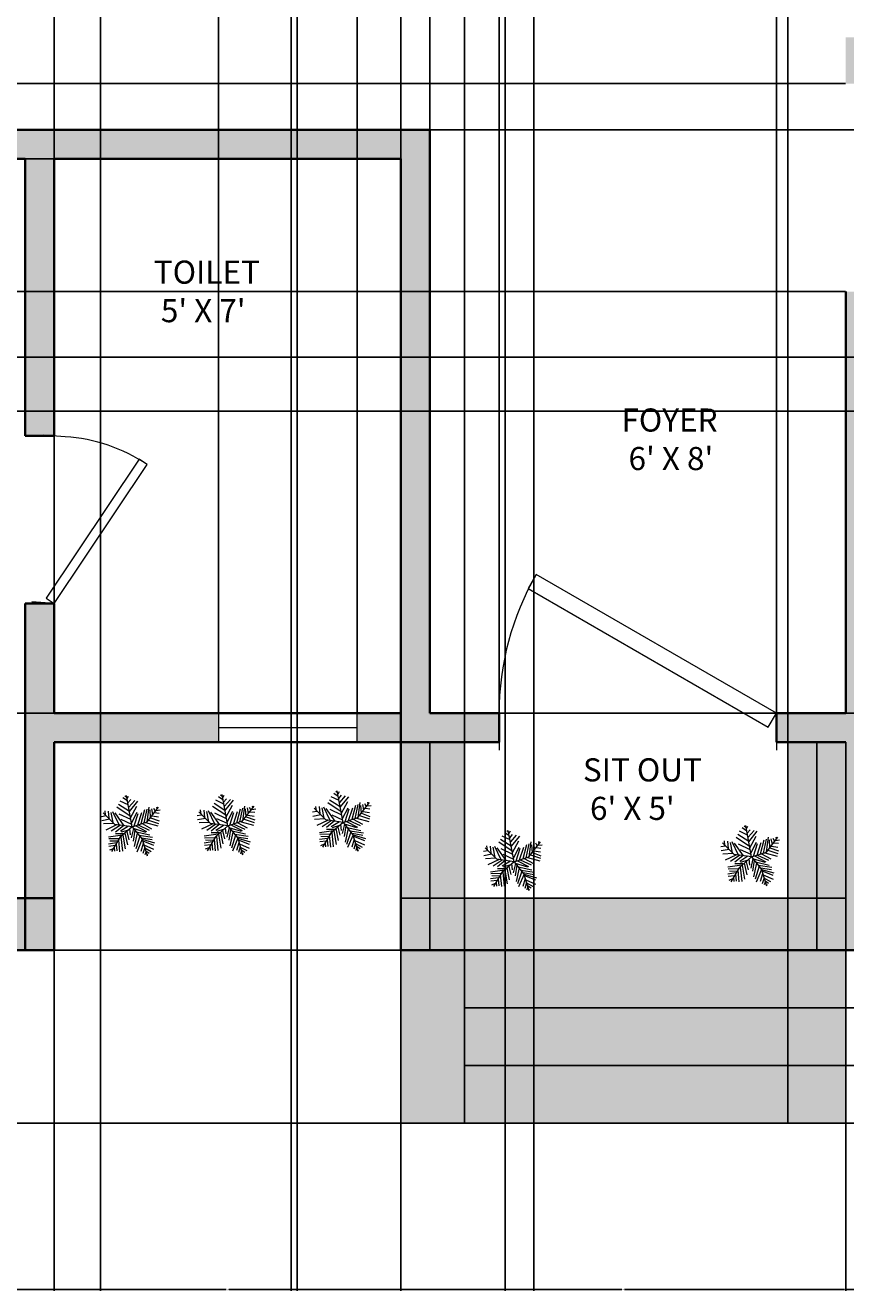
# Model space of a CAD drawing. Units: inches. Extents: x -28 to 649, y -11 to 509.
# Tile 2 of 7: x 204 to 346, y -11 to 208. Entities that reach past the tile are written whole.
import ezdxf

# ---------------------------------------------------------------- set-up
doc = ezdxf.new("R2010")
doc.units = ezdxf.units.IN
doc.header["$MEASUREMENT"] = 0
for name, color, linetype, lineweight in [('A-ANNO-DIMS', 2, 'Continuous', 18), ('A-AREA-IDEN', 18, 'Continuous', 18), ('A-FLOR-CURB-PATT', 31, 'Continuous', 13), ('A-FLOR-STRS', 7, 'Continuous', 25), ('A-FLOR-STRS-PATT', 254, 'Continuous', 13), ('A-WALL', 7, 'Continuous', 35), ('A-WALL-PATT', 251, 'Continuous', 13), ('doors', 40, 'Continuous', 20), ('L-PLNT', 90, 'Continuous', 13), ('window', 30, 'Continuous', 18)]:
    doc.layers.add(name, color=color, linetype=linetype, lineweight=lineweight)
doc.styles.get("Standard").update_dxf_attribs({"font": 'arial.ttf'})
doc.dimstyles.get("Standard").update_dxf_attribs({"dimtxt": 0.18, "dimasz": 0.18, "dimexe": 0.18, "dimexo": 0.0625, "dimgap": 0.09, "dimtad": 0, "dimtih": 1, "dimtoh": 1, "dimdec": 4, "dimzin": 0, "dimdsep": 46, "dimtxsty": 'Standard', "dimcen": 0.09, "dimadec": 0, "dimazin": 0, "dimtfac": 1, "dimtdec": 4, "dimtofl": 0, "dimtmove": 0, "dimatfit": 3, "dimfxl": 1, "dimtolj": 1, "dimtzin": 0, "dimarcsym": 0})

# ---------------------------------------------------------------- blocks, each defined once
blk = doc.blocks.new('*U10')
for p, q in [((0, 0), (0, 100)), ((750, 0), (750, 100))]:
    blk.add_line(p, q)
blk.add_lwpolyline([(0, 0), (649.5, -375), (671.4, -337.1), (21.9, 37.9)], close=True)
blk.add_arc((0, 0), 750, 330, 0)
blk = doc.blocks.new('*U2')
for p, q in [((-185.1152, 1008.5578), (-553.1612, 1185.4942)), ((-221.9198, 1197.3052), (-433.5526, 1338.8594)), ((-258.7244, 1362.456), (-332.3336, 1421.4348)), ((0, 0), (-266.7, 1447.8)), ((-231.1146, 1315.2628), (-166.7002, 1421.4348)), ((-194.31, 1102.9442), (-65.4812, 1256.284)), ((-148.3106, 914.1968), (118.5418, 1220.9018)), ((-129.8956, 701.8528), (265.7602, 1185.4942)), ((-800.1, 114.3), (-1333.5, 647.7)), ((-1234.059, 536.7274), (-1252.4486, 737.2604)), ((-1105.2302, 725.4494), (-1077.6458, 395.1732)), ((-976.4268, 666.4706), (-884.4026, 194.6402)), ((-902.8176, 713.6638), (-617.5756, 100.2538)), ((-369.1382, 53.086), (-783.1836, 642.874)), ((-93.091, 489.5342), (-700.3796, 902.3858)), ((-129.8956, 713.6638), (-626.7704, 1032.1544)), ((-617.5756, 607.4918), (-74.7014, 347.98)), ((-74.7014, 418.7444), (219.7608, 961.39)), ((-28.6766, 171.0436), (228.9556, 678.2816)), ((100.1268, 41.275), (284.1498, 619.2774)), ((256.5654, 88.4682), (449.7832, 666.4706)), ((412.9786, 147.447), (587.8068, 796.2392)), ((560.197, 182.8292), (698.2206, 819.8358)), ((685.8, 228.6), (1219.2, 914.4)), ((689.0258, 230.0224), (790.2448, 914.1968)), ((808.6344, 784.4282), (827.0494, 418.7444)), ((891.4384, 831.6214), (946.658, 572.1096)), ((983.4626, 867.0036), (1066.2666, 725.4494)), ((1029.462, 654.685), (1241.0948, 631.0884)), ((1112.2914, 760.8316), (1296.3144, 784.4282)), ((1121.4862, 925.9824), (1149.0706, 831.6214)), ((-1206.4492, 501.3198), (-1418.082, 465.9376)), ((-1031.621, 347.98), (-1399.667, 277.1902)), ((-847.598, 159.2326), (-1326.0578, 135.636)), ((-718.7946, 88.4682), (-1215.644, -147.447)), ((-543.9664, 76.6572), (-967.2066, -206.4512)), ((0, 0), (-800.1, 114.3)), ((-405.9428, 53.086), (-764.794, -241.8334)), ((0, 0), (-571.5, -495.3)), ((-166.7002, 29.4894), (-543.9664, -206.4512)), ((-525.5514, 347.98), (-28.6766, 123.8504)), ((0, 0), (685.8, 228.6)), ((0, 0), (457.2, -571.5)), ((164.5412, 41.275), (661.416, -218.2368)), ((284.1498, 88.4682), (781.0246, -147.447)), ((458.978, 147.447), (891.4384, -88.4682)), ((615.4166, 194.6402), (1185.8752, 41.275)), ((753.4148, 312.5978), (1222.6798, 159.2326)), ((845.439, 418.7444), (1241.0948, 277.1902)), ((919.0482, 501.3198), (1222.6798, 454.152)), ((-442.7474, -383.3876), (-1086.8406, -477.7486)), ((-617.5756, -548.5384), (-1077.6458, -560.324)), ((-571.5, -495.3), (-952.5, -1143)), ((-387.5278, -324.4088), (-764.794, -324.4088)), ((-525.5514, -465.963), (-451.9422, -1126.5408)), ((-166.7002, -147.447), (-507.1618, -253.619)), ((-433.5526, -383.3876), (-323.1134, -1020.3688)), ((-341.5284, -289.0012), (-221.9198, -831.6214)), ((-240.3094, -218.2368), (-157.5054, -595.7062)), ((-120.7008, -88.4682), (-93.091, -371.5766)), ((63.3222, -76.6826), (-37.8714, -513.1308)), ((44.9326, -64.897), (615.4166, -241.8334)), ((127.7366, -159.258), (54.1274, -654.685)), ((228.9556, -289.0012), (90.932, -914.1968)), ((357.759, -430.5554), (164.5412, -1020.3688)), ((192.151, -230.0224), (817.8292, -371.5766)), ((458.978, -572.1096), (210.5406, -1161.923)), ((311.7596, -383.3876), (937.4378, -477.7486)), ((412.9786, -501.3452), (919.0482, -583.9206)), ((457.2, -571.5), (685.8, -1333.5)), ((468.1982, -572.1096), (1029.462, -737.2604)), ((-718.7946, -737.2604), (-1086.8406, -796.2392)), ((-783.1836, -867.029), (-1077.6458, -902.4112)), ((-875.2078, -1008.5832), (-1040.8412, -1079.3476)), ((-681.9646, -666.496), (-1022.4262, -654.685)), ((-829.2084, -937.7934), (-810.7934, -1126.5408)), ((-737.1842, -784.4536), (-709.5744, -1114.7298)), ((-635.9652, -607.5172), (-580.771, -1150.1374)), ((514.1976, -772.6426), (403.7838, -1138.3264)), ((486.5878, -642.8994), (983.4626, -843.4324)), ((578.612, -961.39), (495.7826, -1232.7128)), ((541.8074, -831.6214), (992.6574, -1032.1544)), ((578.612, -973.1756), (873.0488, -1138.3264)), ((624.6114, -1161.923), (587.8068, -1291.6916)), ((624.6114, -1102.9442), (781.0246, -1209.1162)), ((679.8056, -1268.095), (716.6102, -1291.6916))]:
    blk.add_line(p, q)
blk = doc.blocks.new('*D31')
at = {"layer": 'A-ANNO-DIMS', "color": 0, "lineweight": -2, "transparency": 16777216}
for p, q in [((603.51, 479.94), (632.43, 479.94)), ((632.25, 479.76), (632.25, 249.12)), ((632.25, 18.12), (632.25, 248.76)), ((346.51, 17.94), (632.43, 17.94))]:
    blk.add_line(p, q, dxfattribs=at)
at = {"layer": 'A-ANNO-DIMS', "color": 0, "transparency": 16777216}
for points in [[(632.22, 479.76), (632.28, 479.76), (632.25, 479.94)], [(632.22, 18.12), (632.28, 18.12), (632.25, 17.94)]]:
    blk.add_solid(points, dxfattribs=at)
at = {"layer": 'Defpoints', "color": 0, "transparency": 16777216}
for p in [(603.45, 479.94), (632.25, 479.94), (346.45, 17.94)]:
    blk.add_point(p, dxfattribs=at)
at = {"layer": 'A-ANNO-DIMS', "color": 0, "transparency": 16777216, "insert": (632.25, 248.94), "char_height": 0.18, "attachment_point": 5}
blk.add_mtext('\\A1;462', dxfattribs=at)
blk = doc.blocks.new('*D32')
at = {"layer": 'A-ANNO-DIMS', "color": 0, "lineweight": -2, "transparency": 16777216}
for p, q in [((269.39, 47.94), (-1.53, 47.94)), ((-1.35, 47.76), (-1.35, 33.12)), ((-1.35, 18.12), (-1.35, 32.76)), ((269.39, 17.94), (-1.53, 17.94))]:
    blk.add_line(p, q, dxfattribs=at)
at = {"layer": 'A-ANNO-DIMS', "color": 0, "transparency": 16777216}
for points in [[(-1.38, 47.76), (-1.32, 47.76), (-1.35, 47.94)], [(-1.38, 18.12), (-1.32, 18.12), (-1.35, 17.94)]]:
    blk.add_solid(points, dxfattribs=at)
at = {"layer": 'Defpoints', "color": 0, "transparency": 16777216}
for p in [(269.45, 47.94), (-1.35, 17.94), (269.45, 17.94)]:
    blk.add_point(p, dxfattribs=at)
at = {"layer": 'A-ANNO-DIMS', "color": 0, "transparency": 16777216, "insert": (-1.35, 32.94), "char_height": 0.18, "attachment_point": 5}
blk.add_mtext('\\A1;30', dxfattribs=at)
blk = doc.blocks.new('*D33')
at = {"layer": 'A-ANNO-DIMS', "color": 0, "lineweight": -2, "transparency": 16777216}
for p, q in [((280.51, 37.94), (632.43, 37.94)), ((632.25, 37.76), (632.25, 33.12)), ((632.25, 28.12), (632.25, 32.76)), ((280.51, 27.94), (632.43, 27.94))]:
    blk.add_line(p, q, dxfattribs=at)
at = {"layer": 'A-ANNO-DIMS', "color": 0, "transparency": 16777216}
for points in [[(632.22, 37.76), (632.28, 37.76), (632.25, 37.94)], [(632.22, 28.12), (632.28, 28.12), (632.25, 27.94)]]:
    blk.add_solid(points, dxfattribs=at)
at = {"layer": 'Defpoints', "color": 0, "transparency": 16777216}
for p in [(280.45, 37.94), (632.25, 37.94), (280.45, 27.94)]:
    blk.add_point(p, dxfattribs=at)
at = {"layer": 'A-ANNO-DIMS', "color": 0, "transparency": 16777216, "insert": (632.25, 32.94), "char_height": 0.18, "attachment_point": 5}
blk.add_mtext('\\A1;10', dxfattribs=at)
blk = doc.blocks.new('*D34')
at = {"layer": 'A-ANNO-DIMS', "color": 0, "lineweight": -2, "transparency": 16777216}
for p, q in [((280.45, 48), (280.45, 508.92)), ((280.63, 508.74), (308.23, 508.74)), ((336.27, 508.74), (308.67, 508.74)), ((336.45, 48), (336.45, 508.92))]:
    blk.add_line(p, q, dxfattribs=at)
at = {"layer": 'A-ANNO-DIMS', "color": 0, "transparency": 16777216}
for points in [[(280.63, 508.77), (280.63, 508.71), (280.45, 508.74)], [(336.27, 508.77), (336.27, 508.71), (336.45, 508.74)]]:
    blk.add_solid(points, dxfattribs=at)
at = {"layer": 'Defpoints', "color": 0, "transparency": 16777216}
for p in [(336.45, 508.74), (280.45, 47.94), (336.45, 47.94)]:
    blk.add_point(p, dxfattribs=at)
at = {"layer": 'A-ANNO-DIMS', "color": 0, "transparency": 16777216, "insert": (308.45, 508.74), "char_height": 0.18, "attachment_point": 5}
blk.add_mtext('\\A1;56', dxfattribs=at)
blk = doc.blocks.new('*D37')
at = {"layer": 'A-ANNO-DIMS', "color": 0, "lineweight": -2, "transparency": 16777216}
for p, q in [((27.45, 47.88), (27.45, -11.04)), ((209.45, 47.88), (209.45, -11.04)), ((27.63, -10.86), (118.17, -10.86)), ((209.27, -10.86), (118.73, -10.86))]:
    blk.add_line(p, q, dxfattribs=at)
at = {"layer": 'A-ANNO-DIMS', "color": 0, "transparency": 16777216}
for points in [[(27.63, -10.83), (27.63, -10.89), (27.45, -10.86)], [(209.27, -10.83), (209.27, -10.89), (209.45, -10.86)]]:
    blk.add_solid(points, dxfattribs=at)
at = {"layer": 'Defpoints', "color": 0, "transparency": 16777216}
for p in [(27.45, 47.94), (209.45, 47.94), (209.45, -10.86)]:
    blk.add_point(p, dxfattribs=at)
at = {"layer": 'A-ANNO-DIMS', "color": 0, "transparency": 16777216, "insert": (118.45, -10.86), "char_height": 0.18, "attachment_point": 5}
blk.add_mtext('\\A1;182', dxfattribs=at)
blk = doc.blocks.new('*D38')
at = {"layer": 'A-ANNO-DIMS', "color": 0, "lineweight": -2, "transparency": 16777216}
for p, q in [((209.45, 47.88), (209.45, -11.04)), ((269.45, 47.88), (269.45, -11.04)), ((209.63, -10.86), (239.23, -10.86)), ((269.27, -10.86), (239.67, -10.86))]:
    blk.add_line(p, q, dxfattribs=at)
at = {"layer": 'A-ANNO-DIMS', "color": 0, "transparency": 16777216}
for points in [[(209.63, -10.83), (209.63, -10.89), (209.45, -10.86)], [(269.27, -10.83), (269.27, -10.89), (269.45, -10.86)]]:
    blk.add_solid(points, dxfattribs=at)
at = {"layer": 'Defpoints', "color": 0, "transparency": 16777216}
for p in [(209.45, 47.94), (269.45, 47.94), (269.45, -10.86)]:
    blk.add_point(p, dxfattribs=at)
at = {"layer": 'A-ANNO-DIMS', "color": 0, "transparency": 16777216, "insert": (239.45, -10.86), "char_height": 0.18, "attachment_point": 5}
blk.add_mtext('\\A1;60', dxfattribs=at)
blk = doc.blocks.new('*D39')
at = {"layer": 'A-ANNO-DIMS', "color": 0, "lineweight": -2, "transparency": 16777216}
for p, q in [((269.45, 17.88), (269.45, -11.04)), ((346.45, 17.88), (346.45, -11.04)), ((269.63, -10.86), (307.73, -10.86)), ((346.27, -10.86), (308.17, -10.86))]:
    blk.add_line(p, q, dxfattribs=at)
at = {"layer": 'A-ANNO-DIMS', "color": 0, "transparency": 16777216}
for points in [[(269.63, -10.83), (269.63, -10.89), (269.45, -10.86)], [(346.27, -10.83), (346.27, -10.89), (346.45, -10.86)]]:
    blk.add_solid(points, dxfattribs=at)
at = {"layer": 'Defpoints', "color": 0, "transparency": 16777216}
for p in [(269.45, 17.94), (346.45, 17.94), (346.45, -10.86)]:
    blk.add_point(p, dxfattribs=at)
at = {"layer": 'A-ANNO-DIMS', "color": 0, "transparency": 16777216, "insert": (307.95, -10.86), "char_height": 0.18, "attachment_point": 5}
blk.add_mtext('\\A1;77', dxfattribs=at)
blk = doc.blocks.new('*D40')
at = {"layer": 'A-ANNO-DIMS', "color": 0, "lineweight": -2, "transparency": 16777216}
for p, q in [((346.45, 47.88), (346.45, -11.04)), ((379.58, 47.88), (379.58, -11.04)), ((346.63, -10.86), (362.62, -10.86)), ((379.4, -10.86), (363.41, -10.86))]:
    blk.add_line(p, q, dxfattribs=at)
at = {"layer": 'A-ANNO-DIMS', "color": 0, "transparency": 16777216}
for points in [[(346.63, -10.83), (346.63, -10.89), (346.45, -10.86)], [(379.4, -10.83), (379.4, -10.89), (379.58, -10.86)]]:
    blk.add_solid(points, dxfattribs=at)
at = {"layer": 'Defpoints', "color": 0, "transparency": 16777216}
for p in [(346.45, 47.94), (379.58, 47.94), (379.58, -10.86)]:
    blk.add_point(p, dxfattribs=at)
at = {"layer": 'A-ANNO-DIMS', "color": 0, "transparency": 16777216, "insert": (363.01, -10.86), "char_height": 0.18, "attachment_point": 5}
blk.add_mtext('\\A1;33.13', dxfattribs=at)
blk = doc.blocks.new('*D46')
at = {"layer": 'A-ANNO-DIMS', "color": 0, "lineweight": -2, "transparency": 16777216}
for p, q in [((250.45, 470.88), (250.45, -11.04)), ((292.46, 470.88), (292.46, -11.04)), ((250.63, -10.86), (271.08, -10.86)), ((292.28, -10.86), (271.83, -10.86))]:
    blk.add_line(p, q, dxfattribs=at)
at = {"layer": 'A-ANNO-DIMS', "color": 0, "transparency": 16777216}
for points in [[(250.63, -10.83), (250.63, -10.89), (250.45, -10.86)], [(292.28, -10.83), (292.28, -10.89), (292.46, -10.86)]]:
    blk.add_solid(points, dxfattribs=at)
at = {"layer": 'Defpoints', "color": 0, "transparency": 16777216}
for p in [(250.45, 470.94), (292.46, 470.94), (292.46, -10.86)]:
    blk.add_point(p, dxfattribs=at)
at = {"layer": 'A-ANNO-DIMS', "color": 0, "transparency": 16777216, "insert": (271.45, -10.86), "char_height": 0.18, "attachment_point": 5}
blk.add_mtext('\\A1;42.01', dxfattribs=at)
blk = doc.blocks.new('*D52')
at = {"layer": 'A-ANNO-DIMS', "color": 0, "lineweight": -2, "transparency": 16777216}
for p, q in [((594.39, 262.25), (-1.53, 262.25)), ((-1.35, 262.07), (-1.35, 206.61)), ((-1.35, 150.79), (-1.35, 206.25)), ((594.39, 150.61), (-1.53, 150.61))]:
    blk.add_line(p, q, dxfattribs=at)
at = {"layer": 'A-ANNO-DIMS', "color": 0, "transparency": 16777216}
for points in [[(-1.38, 262.07), (-1.32, 262.07), (-1.35, 262.25)], [(-1.38, 150.79), (-1.32, 150.79), (-1.35, 150.61)]]:
    blk.add_solid(points, dxfattribs=at)
at = {"layer": 'Defpoints', "color": 0, "transparency": 16777216}
for p in [(-1.35, 262.25), (594.45, 262.25), (594.45, 150.61)]:
    blk.add_point(p, dxfattribs=at)
at = {"layer": 'A-ANNO-DIMS', "color": 0, "transparency": 16777216, "insert": (-1.35, 206.43), "char_height": 0.18, "attachment_point": 5}
blk.add_mtext('\\A1;111.64', dxfattribs=at)
blk = doc.blocks.new('*D53')
at = {"layer": 'A-ANNO-DIMS', "color": 0, "lineweight": -2, "transparency": 16777216}
for p, q in [((36.51, 241.9), (632.43, 241.9)), ((632.25, 241.72), (632.25, 191.76)), ((632.25, 141.44), (632.25, 191.39)), ((36.51, 141.26), (632.43, 141.26))]:
    blk.add_line(p, q, dxfattribs=at)
at = {"layer": 'A-ANNO-DIMS', "color": 0, "transparency": 16777216}
for points in [[(632.22, 241.72), (632.28, 241.72), (632.25, 241.9)], [(632.22, 141.44), (632.28, 141.44), (632.25, 141.26)]]:
    blk.add_solid(points, dxfattribs=at)
at = {"layer": 'Defpoints', "color": 0, "transparency": 16777216}
for p in [(36.45, 241.9), (632.25, 241.9), (36.45, 141.26)]:
    blk.add_point(p, dxfattribs=at)
at = {"layer": 'A-ANNO-DIMS', "color": 0, "transparency": 16777216, "insert": (632.25, 191.58), "char_height": 0.18, "attachment_point": 5}
blk.add_mtext('\\A1;100.64', dxfattribs=at)
blk = doc.blocks.new('*D56')
at = {"layer": 'A-ANNO-DIMS', "color": 0, "lineweight": -2, "transparency": 16777216}
for p, q in [((286.45, 89), (286.45, 508.92)), ((286.63, 508.74), (310.23, 508.74)), ((334.27, 508.74), (310.67, 508.74)), ((334.45, 89), (334.45, 508.92))]:
    blk.add_line(p, q, dxfattribs=at)
at = {"layer": 'A-ANNO-DIMS', "color": 0, "transparency": 16777216}
for points in [[(286.63, 508.77), (286.63, 508.71), (286.45, 508.74)], [(334.27, 508.77), (334.27, 508.71), (334.45, 508.74)]]:
    blk.add_solid(points, dxfattribs=at)
at = {"layer": 'Defpoints', "color": 0, "transparency": 16777216}
for p in [(334.45, 508.74), (286.45, 88.94), (334.45, 88.94)]:
    blk.add_point(p, dxfattribs=at)
at = {"layer": 'A-ANNO-DIMS', "color": 0, "transparency": 16777216, "insert": (310.45, 508.74), "char_height": 0.18, "attachment_point": 5}
blk.add_mtext('\\A1;48', dxfattribs=at)
blk = doc.blocks.new('*D59')
at = {"layer": 'A-ANNO-DIMS', "color": 0, "lineweight": -2, "transparency": 16777216}
for p, q in [((346.39, 197.94), (-1.53, 197.94)), ((-1.35, 197.76), (-1.35, 180.12)), ((-1.35, 162.12), (-1.35, 179.76)), ((346.39, 161.94), (-1.53, 161.94))]:
    blk.add_line(p, q, dxfattribs=at)
at = {"layer": 'A-ANNO-DIMS', "color": 0, "transparency": 16777216}
for points in [[(-1.38, 197.76), (-1.32, 197.76), (-1.35, 197.94)], [(-1.38, 162.12), (-1.32, 162.12), (-1.35, 161.94)]]:
    blk.add_solid(points, dxfattribs=at)
at = {"layer": 'Defpoints', "color": 0, "transparency": 16777216}
for p in [(-1.35, 197.94), (346.45, 197.94), (346.45, 161.94)]:
    blk.add_point(p, dxfattribs=at)
at = {"layer": 'A-ANNO-DIMS', "color": 0, "transparency": 16777216, "insert": (-1.35, 179.94), "char_height": 0.18, "attachment_point": 5}
blk.add_mtext('\\A1;36', dxfattribs=at)
blk = doc.blocks.new('*D61')
at = {"layer": 'A-ANNO-DIMS', "color": 0, "lineweight": -2, "transparency": 16777216}
for p, q in [((274.51, 189.94), (632.43, 189.94)), ((632.25, 189.76), (632.25, 139.62)), ((632.25, 89.12), (632.25, 139.26)), ((274.51, 88.94), (632.43, 88.94))]:
    blk.add_line(p, q, dxfattribs=at)
at = {"layer": 'A-ANNO-DIMS', "color": 0, "transparency": 16777216}
for points in [[(632.22, 189.76), (632.28, 189.76), (632.25, 189.94)], [(632.22, 89.12), (632.28, 89.12), (632.25, 88.94)]]:
    blk.add_solid(points, dxfattribs=at)
at = {"layer": 'Defpoints', "color": 0, "transparency": 16777216}
for p in [(274.45, 189.94), (632.25, 189.94), (274.45, 88.94)]:
    blk.add_point(p, dxfattribs=at)
at = {"layer": 'A-ANNO-DIMS', "color": 0, "transparency": 16777216, "insert": (632.25, 139.44), "char_height": 0.18, "attachment_point": 5}
blk.add_mtext('\\A1;101', dxfattribs=at)
blk = doc.blocks.new('*D62')
at = {"layer": 'A-ANNO-DIMS', "color": 0, "lineweight": -2, "transparency": 16777216}
for p, q in [((188.45, 381.88), (188.45, -11.04)), ((217.45, 381.88), (217.45, -11.04)), ((188.63, -10.86), (202.73, -10.86)), ((217.27, -10.86), (203.17, -10.86))]:
    blk.add_line(p, q, dxfattribs=at)
at = {"layer": 'A-ANNO-DIMS', "color": 0, "transparency": 16777216}
for points in [[(188.63, -10.83), (188.63, -10.89), (188.45, -10.86)], [(217.27, -10.83), (217.27, -10.89), (217.45, -10.86)]]:
    blk.add_solid(points, dxfattribs=at)
at = {"layer": 'Defpoints', "color": 0, "transparency": 16777216}
for p in [(188.45, 381.94), (217.45, 381.94), (217.45, -10.86)]:
    blk.add_point(p, dxfattribs=at)
at = {"layer": 'A-ANNO-DIMS', "color": 0, "transparency": 16777216, "insert": (202.95, -10.86), "char_height": 0.18, "attachment_point": 5}
blk.add_mtext('\\A1;29', dxfattribs=at)
blk = doc.blocks.new('*D64')
at = {"layer": 'A-ANNO-DIMS', "color": 0, "lineweight": -2, "transparency": 16777216}
for p, q in [((251.52, 333.88), (251.52, -11.04)), ((287.52, 333.88), (287.52, -11.04)), ((251.7, -10.86), (269.3, -10.86)), ((287.34, -10.86), (269.74, -10.86))]:
    blk.add_line(p, q, dxfattribs=at)
at = {"layer": 'A-ANNO-DIMS', "color": 0, "transparency": 16777216}
for points in [[(251.7, -10.83), (251.7, -10.89), (251.52, -10.86)], [(287.34, -10.83), (287.34, -10.89), (287.52, -10.86)]]:
    blk.add_solid(points, dxfattribs=at)
at = {"layer": 'Defpoints', "color": 0, "transparency": 16777216}
for p in [(251.52, 333.94), (287.52, 333.94), (287.52, -10.86)]:
    blk.add_point(p, dxfattribs=at)
at = {"layer": 'A-ANNO-DIMS', "color": 0, "transparency": 16777216, "insert": (269.52, -10.86), "char_height": 0.18, "attachment_point": 5}
blk.add_mtext('\\A1;36', dxfattribs=at)
blk = doc.blocks.new('*D73')
at = {"layer": 'A-ANNO-DIMS', "color": 0, "lineweight": -2, "transparency": 16777216}
for p, q in [((269.39, 184.94), (-1.53, 184.94)), ((-1.35, 184.76), (-1.35, 137.12)), ((-1.35, 89.12), (-1.35, 136.76)), ((269.39, 88.94), (-1.53, 88.94))]:
    blk.add_line(p, q, dxfattribs=at)
at = {"layer": 'A-ANNO-DIMS', "color": 0, "transparency": 16777216}
for points in [[(-1.38, 184.76), (-1.32, 184.76), (-1.35, 184.94)], [(-1.38, 89.12), (-1.32, 89.12), (-1.35, 88.94)]]:
    blk.add_solid(points, dxfattribs=at)
at = {"layer": 'Defpoints', "color": 0, "transparency": 16777216}
for p in [(-1.35, 184.94), (269.45, 184.94), (269.45, 88.94)]:
    blk.add_point(p, dxfattribs=at)
at = {"layer": 'A-ANNO-DIMS', "color": 0, "transparency": 16777216, "insert": (-1.35, 136.94), "char_height": 0.18, "attachment_point": 5}
blk.add_mtext('\\A1;96', dxfattribs=at)
blk = doc.blocks.new('*D74')
at = {"layer": 'A-ANNO-DIMS', "color": 0, "lineweight": -2, "transparency": 16777216}
for p, q in [((237.88, 89), (237.88, 508.92)), ((238.06, 508.74), (249.66, 508.74)), ((261.7, 508.74), (250.1, 508.74)), ((261.88, 89), (261.88, 508.92))]:
    blk.add_line(p, q, dxfattribs=at)
at = {"layer": 'A-ANNO-DIMS', "color": 0, "transparency": 16777216}
for points in [[(238.06, 508.77), (238.06, 508.71), (237.88, 508.74)], [(261.7, 508.77), (261.7, 508.71), (261.88, 508.74)]]:
    blk.add_solid(points, dxfattribs=at)
at = {"layer": 'Defpoints', "color": 0, "transparency": 16777216}
for p in [(261.88, 508.74), (237.88, 88.94), (261.88, 88.94)]:
    blk.add_point(p, dxfattribs=at)
at = {"layer": 'A-ANNO-DIMS', "color": 0, "transparency": 16777216, "insert": (249.88, 508.74), "char_height": 0.18, "attachment_point": 5}
blk.add_mtext('\\A1;24', dxfattribs=at)
blk = doc.blocks.new('*D75')
at = {"layer": 'A-ANNO-DIMS', "color": 0, "lineweight": -2, "transparency": 16777216}
for p, q in [((209.45, 89), (209.45, 508.92)), ((209.63, 508.74), (223.27, 508.74)), ((237.7, 508.74), (224.06, 508.74)), ((237.88, 89), (237.88, 508.92))]:
    blk.add_line(p, q, dxfattribs=at)
at = {"layer": 'A-ANNO-DIMS', "color": 0, "transparency": 16777216}
for points in [[(209.63, 508.77), (209.63, 508.71), (209.45, 508.74)], [(237.7, 508.77), (237.7, 508.71), (237.88, 508.74)]]:
    blk.add_solid(points, dxfattribs=at)
at = {"layer": 'Defpoints', "color": 0, "transparency": 16777216}
for p in [(237.88, 508.74), (209.45, 88.94), (237.88, 88.94)]:
    blk.add_point(p, dxfattribs=at)
at = {"layer": 'A-ANNO-DIMS', "color": 0, "transparency": 16777216, "insert": (223.66, 508.74), "char_height": 0.18, "attachment_point": 5}
blk.add_mtext('\\A1;28.43', dxfattribs=at)
blk = doc.blocks.new('*D76')
at = {"layer": 'A-ANNO-DIMS', "color": 0, "lineweight": -2, "transparency": 16777216}
for p, q in [((269.45, 185), (269.45, 508.92)), ((269.63, 508.74), (271.8, 508.74)), ((274.27, 508.74), (272.1, 508.74)), ((274.45, 190), (274.45, 508.92))]:
    blk.add_line(p, q, dxfattribs=at)
at = {"layer": 'A-ANNO-DIMS', "color": 0, "transparency": 16777216}
for points in [[(269.63, 508.77), (269.63, 508.71), (269.45, 508.74)], [(274.27, 508.77), (274.27, 508.71), (274.45, 508.74)]]:
    blk.add_solid(points, dxfattribs=at)
at = {"layer": 'Defpoints', "color": 0, "transparency": 16777216}
for p in [(274.45, 508.74), (274.45, 189.94), (269.45, 184.94)]:
    blk.add_point(p, dxfattribs=at)
at = {"layer": 'A-ANNO-DIMS', "color": 0, "transparency": 16777216, "insert": (271.95, 508.74), "char_height": 0.18, "attachment_point": 5}
blk.add_mtext('\\A1;5', dxfattribs=at)

msp = doc.modelspace()

# ---------------------------------------------------------------- hatches: boundary and pattern name
at = {"layer": 'A-FLOR-CURB-PATT'}
h = msp.add_hatch(color=256, dxfattribs=at)
h.dxf.hatch_style = 1
h.paths.add_polyline_path([(274.4499, 83.9382), (269.4499, 83.9382), (269.4499, 56.9382), (274.4499, 56.9382)])
h.paths.add_polyline_path([(280.4499, 83.9382), (274.4499, 83.9382), (274.4499, 56.9382), (280.4499, 56.9382)])
h.paths.add_polyline_path([(280.4499, 56.9382), (274.4499, 56.9382), (274.4499, 47.9382), (280.4499, 47.9382)])
h.paths.add_polyline_path([(274.4499, 56.9382), (269.4499, 56.9382), (269.4499, 47.9382), (274.4499, 47.9382)])
h.paths.add_polyline_path([(341.4499, 56.9382), (336.4499, 56.9382), (336.4499, 47.9382), (341.4499, 47.9382)])
h.paths.add_polyline_path([(341.4499, 83.9382), (336.4499, 83.9382), (336.4499, 56.9382), (341.4499, 56.9382)])
h.paths.add_polyline_path([(346.4499, 83.9382), (341.4499, 83.9382), (341.4499, 56.9382), (346.4499, 56.9382)])
h.paths.add_polyline_path([(346.4499, 56.9382), (341.4499, 56.9382), (341.4499, 47.9382), (346.4499, 47.9382)])
h = msp.add_hatch(color=256, dxfattribs=at)
h.dxf.hatch_style = 1
h.paths.add_polyline_path([(280.4499, 47.9382), (269.4499, 47.9382), (269.4499, 17.9382), (280.4499, 17.9382)])
h.paths.add_polyline_path([(346.4499, 47.9382), (336.4499, 47.9382), (336.4499, 17.9382), (346.4499, 17.9382)])
at = {"layer": 'A-FLOR-STRS-PATT'}
h = msp.add_hatch(color=256, dxfattribs=at)
h.dxf.hatch_style = 1
h.paths.add_polyline_path([(336.4499, 56.9382), (280.4499, 56.9382), (280.4499, 47.9382), (336.4499, 47.9382)])
h.paths.add_polyline_path([(336.4499, 47.9382), (280.4499, 47.9382), (280.4499, 37.9382), (336.4499, 37.9382)])
h.paths.add_polyline_path([(336.4499, 37.9382), (280.4499, 37.9382), (280.4499, 27.9382), (336.4499, 27.9382)])
h.paths.add_polyline_path([(336.4499, 27.9382), (280.4499, 27.9382), (280.4499, 17.9382), (336.4499, 17.9382)])
at = {"layer": 'A-WALL-PATT'}
h = msp.add_hatch(color=256, dxfattribs=at)
h.dxf.hatch_style = 1
h.paths.add_polyline_path([(603.4499, 102.6102), (594.4499, 102.6102), (594.4499, 56.9382), (520.6175, 56.9382), (520.6175, 47.9382), (603.4499, 47.9382)])
h.paths.add_polyline_path([(484.6175, 56.9382), (476.4499, 56.9382), (476.4499, 200.9382), (479.4499, 200.9382), (479.4499, 205.9382), (346.4499, 205.9382), (346.4499, 197.9382), (351.4499, 197.9382), (351.4499, 200.9382), (471.4499, 200.9382), (471.4499, 56.9382), (415.5771, 56.9382), (415.5771, 47.9382), (484.6175, 47.9382)])
h.paths.add_polyline_path([(379.5771, 56.9382), (351.4499, 56.9382), (351.4499, 161.9382), (346.4499, 161.9382), (346.4499, 88.9382), (334.4499, 88.9382), (334.4499, 83.9382), (346.4499, 83.9382), (346.4499, 47.9382), (379.5771, 47.9382)])
h = msp.add_hatch(color=256, dxfattribs=at)
h.dxf.hatch_style = 1
h.paths.add_polyline_path([(131.1226, 56.9382), (36.4499, 56.9382), (36.4499, 93.2558), (27.4499, 93.2558), (27.4499, 47.9382), (131.1226, 47.9382)])
h.paths.add_polyline_path([(204.4499, 56.9382), (167.1226, 56.9382), (167.1226, 47.9382), (204.4499, 47.9382)])
h.paths.add_polyline_path([(209.4499, 56.9382), (204.4499, 56.9382), (204.4499, 47.9382), (209.4499, 47.9382)])
h.paths.add_polyline_path([(209.4499, 83.9382), (237.8774, 83.9382), (237.8774, 88.9382), (209.4499, 88.9382), (209.4499, 107.9382), (204.4499, 107.9382), (204.4499, 56.9382), (209.4499, 56.9382)])
h.paths.add_polyline_path([(269.4499, 88.9382), (261.8774, 88.9382), (261.8774, 83.9382), (269.4499, 83.9382)], flags=17)
h.paths.add_polyline_path([(274.4499, 189.9382), (201.4499, 189.9382), (201.4499, 184.9382), (204.4499, 184.9382), (204.4499, 136.9382), (209.4499, 136.9382), (209.4499, 184.9382), (269.4499, 184.9382), (269.4499, 83.9382), (286.4499, 83.9382), (286.4499, 88.9382), (274.4499, 88.9382)])

# ---------------------------------------------------------------- linework, layer by layer
at = {"layer": 'A-FLOR-STRS'}
for p, q in [((274.4499, 47.9382), (274.4499, 83.9382)), ((280.4499, 47.9382), (280.4499, 83.9382)), ((336.4499, 47.9382), (336.4499, 83.9382)), ((341.4499, 47.9382), (341.4499, 83.9382)), ((346.4499, 47.9382), (346.4499, 83.9382)), ((346.4499, 56.9382), (269.4499, 56.9382)), ((280.4499, 56.9382), (280.4499, 17.9382)), ((269.4499, 47.9382), (269.4499, 17.9382)), ((336.4499, 17.9382), (336.4499, 47.9382)), ((346.4499, 47.9382), (346.4499, 17.9382)), ((280.4499, 37.9382), (336.4499, 37.9382)), ((280.4499, 27.9382), (336.4499, 27.9382)), ((269.4499, 17.9382), (280.4499, 17.9382)), ((280.4499, 17.9382), (336.4499, 17.9382)), ((346.4499, 17.9382), (336.4499, 17.9382))]:
    msp.add_line(p, q, dxfattribs=at)
at = {"layer": 'A-WALL'}
for p, q in [((201.4499, 189.9382), (274.4499, 189.9382)), ((274.4499, 88.9382), (274.4499, 189.9382)), ((201.4499, 184.9382), (204.4499, 184.9382)), ((204.4499, 136.9382), (204.4499, 184.9382)), ((209.4499, 184.9382), (269.4499, 184.9382)), ((209.4499, 136.9382), (209.4499, 184.9382)), ((269.4499, 47.9382), (269.4499, 184.9382)), ((346.4499, 88.9382), (346.4499, 161.9382)), ((204.4499, 136.9382), (209.4499, 136.9382)), ((204.4499, 107.9382), (209.4499, 107.9382)), ((204.4499, 47.9382), (204.4499, 107.9382)), ((209.4499, 88.9382), (209.4499, 107.9382)), ((209.4499, 88.9382), (269.4499, 88.9382)), ((274.4499, 88.9382), (286.4499, 88.9382)), ((286.4499, 83.9382), (286.4499, 88.9382)), ((334.4499, 88.9382), (346.4499, 88.9382)), ((334.4499, 83.9382), (334.4499, 88.9382)), ((209.4499, 83.9382), (286.4499, 83.9382)), ((209.4499, 47.9382), (209.4499, 83.9382)), ((334.4499, 83.9382), (346.4499, 83.9382)), ((209.4499, 56.9382), (36.4499, 56.9382))]:
    msp.add_line(p, q, dxfattribs=at)
msp.add_lwpolyline([(209.4499, 47.9382), (27.4499, 47.9382), (27.4499, 479.9382), (603.4499, 479.9382), (603.4499, 47.9382), (269.4499, 47.9382)], dxfattribs=at)
at = {"layer": 'window'}
for p, q in [((237.8774, 88.9382), (237.8774, 83.9382)), ((261.8774, 88.9382), (237.8774, 88.9382)), ((237.8774, 88.9382), (237.8774, 86.4382)), ((261.8774, 83.9382), (261.8774, 88.9382)), ((237.8774, 86.4382), (261.8774, 86.4382)), ((237.8774, 83.9382), (261.8774, 83.9382))]:
    msp.add_line(p, q, dxfattribs=at)

# ---------------------------------------------------------------- block references
at = {"layer": 'doors'}
for p, xscale, yscale, zscale, rotation in [((209.4499, 107.9382), 0.0385810261037888, 0.0385810261037888, 0.0385810261037888, 86.1859251657114), ((334.4499, 88.9382), 0.0639999999999986, 0.0639999999999986, 0.0639999999999986, 180)]:
    msp.add_blockref('*U10', p, dxfattribs=dict(at, xscale=xscale, yscale=yscale, zscale=zscale, rotation=rotation))
at = {"layer": 'L-PLNT', "xscale": 0.00375069843307, "yscale": 0.00375069843307, "zscale": 0.00375069843307}
for p in [(222.9422, 69.2672), (239.496, 69.4218), (259.4535, 70.0403), (289.0523, 63.2271), (330.1454, 64.0494)]:
    msp.add_blockref('*U2', p, dxfattribs=at)

# ---------------------------------------------------------------- texts
at = {"layer": 'A-AREA-IDEN', "char_height": 4, "attachment_point": 1}
for s, width, insert in [("TOILET\\P 5' X 7'", 33.096465, (226.69, 167.3045)), ("FOYER\\P 6' X 8'", 46.696275, (307.6391, 141.6972)), ("SIT OUT\\P 6' X 5'", 46.696275, (300.9685, 81.1299))]:
    msp.add_mtext_dynamic_manual_height_columns(s, width=width, gutter_width=1, heights=[0], dxfattribs=dict(at, insert=insert))

# ---------------------------------------------------------------- dimensions: what is measured, and where the dimension line sits
at = {"layer": 'A-ANNO-DIMS'}
for base, p1, p2, override, picture, middle in [((237.8774, 508.7392), (209.4499, 88.9382), (237.8774, 88.9382), {"dimdec": 2, "dimlfac": 1, "dimrnd": 0, "dimzin": 0, "dimdsep": 46, "dimlunit": 2}, '*D75', (223.6637, 508.7392)), ((261.8774, 508.7392), (237.8774, 88.9382), (261.8774, 88.9382), {"dimdec": 0, "dimlfac": 1, "dimrnd": 0, "dimzin": 0, "dimdsep": 46, "dimlunit": 2}, '*D74', (249.8774, 508.7392)), ((274.4499, 508.7392), (269.4499, 184.9382), (274.4499, 189.9382), {"dimdec": 0, "dimlfac": 1, "dimrnd": 0, "dimzin": 0, "dimdsep": 46, "dimlunit": 2}, '*D76', (271.9499, 508.7392)), ((336.4499, 508.7392), (280.4499, 47.9382), (336.4499, 47.9382), {"dimdec": 0, "dimlfac": 1, "dimrnd": 0, "dimzin": 0, "dimdsep": 46, "dimlunit": 2}, '*D34', (308.4499, 508.7392)), ((334.4499, 508.7392), (286.4499, 88.9382), (334.4499, 88.9382), {"dimdec": 0, "dimlfac": 1, "dimrnd": 0, "dimzin": 0, "dimdsep": 46, "dimlunit": 2}, '*D56', (310.4499, 508.7392)), ((292.4601, -10.8628), (250.4499, 470.9382), (292.4601, 470.9382), {"dimdec": 2, "dimlfac": 1, "dimrnd": 0, "dimzin": 0, "dimdsep": 46, "dimlunit": 2}, '*D46', (271.455, -10.8628)), ((217.4499, -10.8628), (188.4499, 381.9382), (217.4499, 381.9382), {"dimdec": 0, "dimlfac": 1, "dimrnd": 0, "dimzin": 0, "dimdsep": 46, "dimlunit": 2}, '*D62', (202.9499, -10.8628)), ((287.5222, -10.8628), (251.5222, 333.9382), (287.5222, 333.9382), {"dimdec": 0, "dimlfac": 1, "dimrnd": 0, "dimzin": 0, "dimdsep": 46, "dimlunit": 2}, '*D64', (269.5222, -10.8628)), ((209.4499, -10.8628), (27.4499, 47.9382), (209.4499, 47.9382), {"dimdec": 0, "dimlfac": 1, "dimrnd": 0, "dimzin": 0, "dimdsep": 46, "dimlunit": 2}, '*D37', (118.4499, -10.8628)), ((269.4499, -10.8628), (209.4499, 47.9382), (269.4499, 47.9382), {"dimdec": 0, "dimlfac": 1, "dimrnd": 0, "dimzin": 0, "dimdsep": 46, "dimlunit": 2}, '*D38', (239.4499, -10.8628)), ((379.5771, -10.8628), (346.4499, 47.9382), (379.5771, 47.9382), {"dimdec": 2, "dimlfac": 1, "dimrnd": 0, "dimzin": 0, "dimdsep": 46, "dimlunit": 2}, '*D40', (363.0135, -10.8628)), ((346.4499, -10.8628), (269.4499, 17.9382), (346.4499, 17.9382), {"dimdec": 0, "dimlfac": 1, "dimrnd": 0, "dimzin": 0, "dimdsep": 46, "dimlunit": 2}, '*D39', (307.9499, -10.8628))]:
    dim = msp.add_linear_dim(base=base, p1=p1, p2=p2, dimstyle='Standard', override=override, dxfattribs=at)
    dim.commit()
    dim.dimension.update_dxf_attribs({"geometry": picture, "text_midpoint": middle})
for base, p1, p2, override, picture, middle in [((632.2509, 479.9382), (346.4499, 17.9382), (603.4499, 479.9382), {"dimdec": 0, "dimlfac": 1, "dimrnd": 0, "dimzin": 0, "dimdsep": 46, "dimlunit": 2}, '*D31', (632.2509, 248.9382)), ((-1.3511, 262.2528), (594.4499, 150.6102), (594.4499, 262.2528), {"dimdec": 2, "dimlfac": 1, "dimrnd": 0, "dimzin": 0, "dimdsep": 46, "dimlunit": 2}, '*D52', (-1.3511, 206.4315)), ((632.2509, 241.898), (36.4499, 141.2558), (36.4499, 241.898), {"dimdec": 2, "dimlfac": 1, "dimrnd": 0, "dimzin": 0, "dimdsep": 46, "dimlunit": 2}, '*D53', (632.2509, 191.5769)), ((-1.3511, 197.9382), (346.4499, 161.9382), (346.4499, 197.9382), {"dimdec": 0, "dimlfac": 1, "dimrnd": 0, "dimzin": 0, "dimdsep": 46, "dimlunit": 2}, '*D59', (-1.3511, 179.9382)), ((632.2509, 189.9382), (274.4499, 88.9382), (274.4499, 189.9382), {"dimdec": 0, "dimlfac": 1, "dimrnd": 0, "dimzin": 0, "dimdsep": 46, "dimlunit": 2}, '*D61', (632.2509, 139.4382)), ((-1.3511, 184.9382), (269.4499, 88.9382), (269.4499, 184.9382), {"dimdec": 0, "dimlfac": 1, "dimrnd": 0, "dimzin": 0, "dimdsep": 46, "dimlunit": 2}, '*D73', (-1.3511, 136.9382)), ((-1.3511, 17.9382), (269.4499, 47.9382), (269.4499, 17.9382), {"dimdec": 0, "dimlfac": 1, "dimrnd": 0, "dimzin": 0, "dimdsep": 46, "dimlunit": 2}, '*D32', (-1.3511, 32.9382)), ((632.2509, 37.9382), (280.4499, 27.9382), (280.4499, 37.9382), {"dimdec": 0, "dimlfac": 1, "dimrnd": 0, "dimzin": 0, "dimdsep": 46, "dimlunit": 2}, '*D33', (632.2509, 32.9382))]:
    dim = msp.add_linear_dim(base=base, p1=p1, p2=p2, angle=90, dimstyle='Standard', override=override, dxfattribs=at)
    dim.commit()
    dim.dimension.update_dxf_attribs({"geometry": picture, "text_midpoint": middle})

doc.saveas('drawing.dxf')
